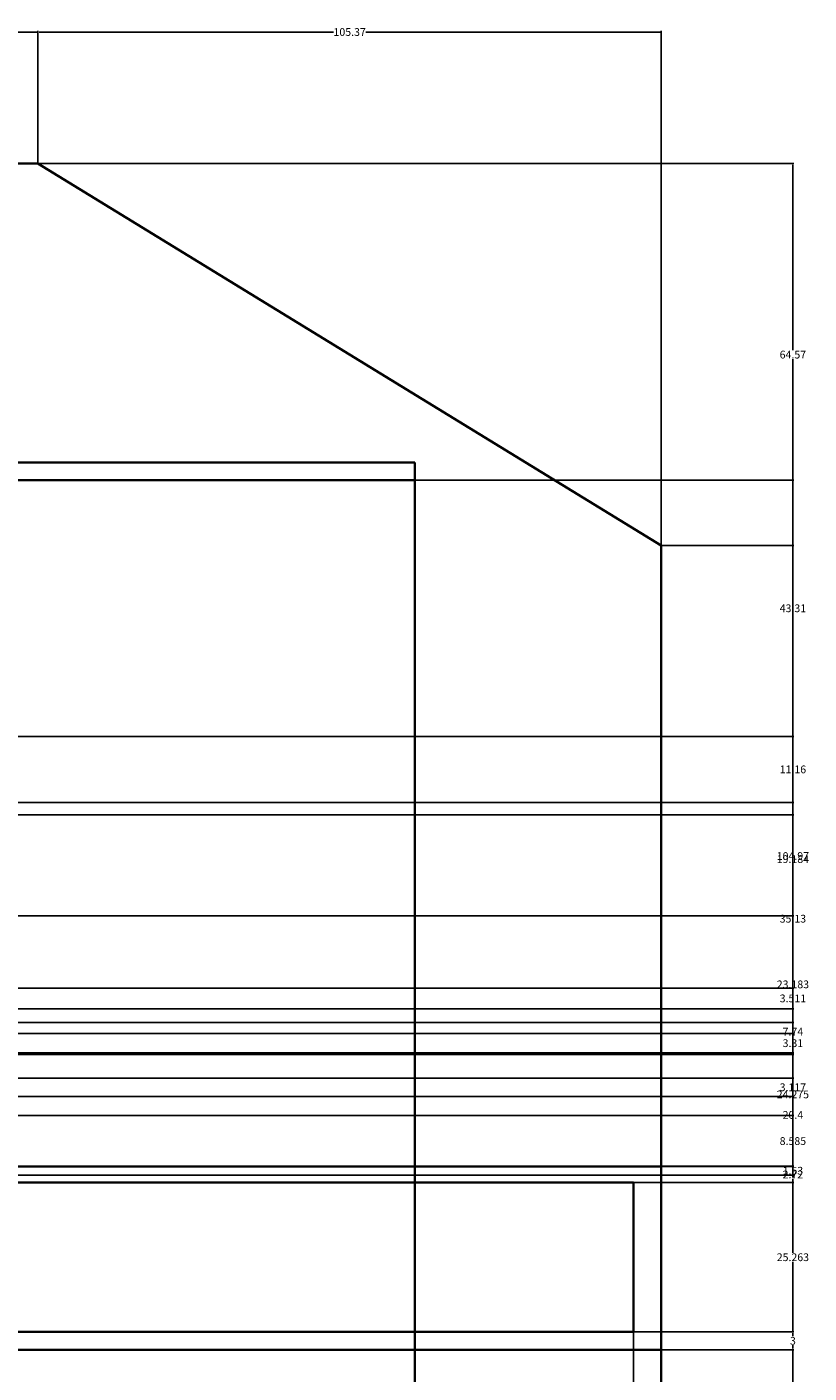
# Model space of a CAD drawing. Units: inches. Extents: x 30 to 515, y 94 to 489.
# Tile 7 of 7: x 383 to 515, y 262 to 489. Entities that reach past the tile are written whole.
import ezdxf

# ---------------------------------------------------------------- set-up
doc = ezdxf.new("R2010")
doc.units = ezdxf.units.IN
doc.header["$MEASUREMENT"] = 0
for name, color, linetype, lineweight in [('A-ANNO-DIMS', 2, 'Continuous', 18), ('A-ROOF', 1, 'Continuous', 35), ('A-WALL', 7, 'Continuous', 35)]:
    doc.layers.add(name, color=color, linetype=linetype, lineweight=lineweight)
doc.styles.get("Standard").update_dxf_attribs({"font": 'arial.ttf'})
doc.dimstyles.get("Standard").update_dxf_attribs({"dimtxt": 1.3125, "dimasz": 0.18, "dimexe": 0.18, "dimexo": 0.0625, "dimgap": 0.09, "dimtad": 0, "dimtih": 1, "dimtoh": 1, "dimdec": 4, "dimzin": 0, "dimdsep": 46, "dimlunit": 4, "dimtxsty": 'Standard', "dimcen": 0.09, "dimadec": 0, "dimazin": 0, "dimtfac": 1, "dimtdec": 4, "dimtofl": 0, "dimtmove": 0, "dimatfit": 3, "dimfxl": 1, "dimtolj": 1, "dimtzin": 0, "dimarcsym": 0})

# ---------------------------------------------------------------- blocks, each defined once
blk = doc.blocks.new('*D5')
at = {"layer": 'A-ANNO-DIMS', "color": 0, "lineweight": -2, "transparency": 16777216}
for p, q in [((191.21, 466.11), (191.21, 488.48)), ((191.39, 488.3), (285.04, 488.3)), ((384.19, 488.3), (290.54, 488.3)), ((384.37, 466.11), (384.37, 488.48))]:
    blk.add_line(p, q, dxfattribs=at)
at = {"layer": 'A-ANNO-DIMS', "color": 0, "transparency": 16777216}
for points in [[(191.39, 488.33), (191.39, 488.27), (191.21, 488.3)], [(384.19, 488.33), (384.19, 488.27), (384.37, 488.3)]]:
    blk.add_solid(points, dxfattribs=at)
at = {"layer": 'Defpoints', "color": 0, "transparency": 16777216}
for p in [(384.37, 488.3), (191.21, 466.05), (384.37, 466.05)]:
    blk.add_point(p, dxfattribs=at)
at = {"layer": 'A-ANNO-DIMS', "color": 0, "transparency": 16777216, "insert": (287.79, 488.3), "char_height": 1.312, "attachment_point": 5}
blk.add_mtext('\\A1;193.16', dxfattribs=at)
blk = doc.blocks.new('*D6')
at = {"layer": 'A-ANNO-DIMS', "color": 0, "lineweight": -2, "transparency": 16777216}
for p, q in [((384.37, 466.11), (384.37, 488.48)), ((384.55, 488.3), (434.3, 488.3)), ((489.56, 488.3), (439.81, 488.3)), ((489.74, 401.54), (489.74, 488.48))]:
    blk.add_line(p, q, dxfattribs=at)
at = {"layer": 'A-ANNO-DIMS', "color": 0, "transparency": 16777216}
for points in [[(384.55, 488.33), (384.55, 488.27), (384.37, 488.3)], [(489.56, 488.33), (489.56, 488.27), (489.74, 488.3)]]:
    blk.add_solid(points, dxfattribs=at)
at = {"layer": 'Defpoints', "color": 0, "transparency": 16777216}
for p in [(489.74, 488.3), (384.37, 466.05), (489.74, 401.48)]:
    blk.add_point(p, dxfattribs=at)
at = {"layer": 'A-ANNO-DIMS', "color": 0, "transparency": 16777216, "insert": (437.06, 488.3), "char_height": 1.312, "attachment_point": 5}
blk.add_mtext('\\A1;105.37', dxfattribs=at)
blk = doc.blocks.new('*D15')
at = {"layer": 'A-ANNO-DIMS', "color": 0, "lineweight": -2, "transparency": 16777216}
for p, q in [((485.027297, 268.465557), (485.027297, 94.504382)), ((489.742649, 265.465557), (489.742649, 94.504382)), ((484.847297, 94.684382), (484.667297, 94.684382)), ((489.922649, 94.684382), (490.102649, 94.684382))]:
    blk.add_line(p, q, dxfattribs=at)
at = {"layer": 'A-ANNO-DIMS', "color": 0, "transparency": 16777216}
for points in [[(484.847297, 94.714382), (484.847297, 94.654382), (485.027297, 94.684382)], [(489.922649, 94.714382), (489.922649, 94.654382), (489.742649, 94.684382)]]:
    blk.add_solid(points, dxfattribs=at)
at = {"layer": 'Defpoints', "color": 0, "transparency": 16777216}
for p in [(485.027297, 268.528057), (489.742649, 265.528057), (489.742649, 94.684382)]:
    blk.add_point(p, dxfattribs=at)
at = {"layer": 'A-ANNO-DIMS', "color": 0, "transparency": 16777216, "insert": (487.384973, 94.684382), "char_height": 1.3125, "attachment_point": 5}
blk.add_mtext('\\A1;4.715', dxfattribs=at)
blk = doc.blocks.new('*D17')
at = {"layer": 'A-ANNO-DIMS', "color": 0, "lineweight": -2, "transparency": 16777216}
for p, q in [((489.81, 265.53), (512.17, 265.53)), ((511.99, 265.35), (511.99, 253.49)), ((511.99, 240.11), (511.99, 251.97)), ((489.81, 239.93), (512.17, 239.93))]:
    blk.add_line(p, q, dxfattribs=at)
at = {"layer": 'A-ANNO-DIMS', "color": 0, "transparency": 16777216}
for points in [[(511.96, 265.35), (512.02, 265.35), (511.99, 265.53)], [(511.96, 240.11), (512.02, 240.11), (511.99, 239.93)]]:
    blk.add_solid(points, dxfattribs=at)
at = {"layer": 'Defpoints', "color": 0, "transparency": 16777216}
for p in [(489.74, 265.53), (511.99, 265.53), (489.74, 239.93)]:
    blk.add_point(p, dxfattribs=at)
at = {"layer": 'A-ANNO-DIMS', "color": 0, "transparency": 16777216, "insert": (511.99, 252.73), "char_height": 1.312, "attachment_point": 5}
blk.add_mtext('\\A1;25.595', dxfattribs=at)
blk = doc.blocks.new('*D18')
at = {"layer": 'A-ANNO-DIMS', "color": 0, "lineweight": -2, "transparency": 16777216}
for p, q in [((485.09, 268.53), (512.17, 268.53)), ((511.99, 268.35), (511.99, 267.79)), ((489.81, 265.53), (512.17, 265.53)), ((511.99, 265.71), (511.99, 266.27))]:
    blk.add_line(p, q, dxfattribs=at)
at = {"layer": 'A-ANNO-DIMS', "color": 0, "transparency": 16777216}
for points in [[(511.96, 268.35), (512.02, 268.35), (511.99, 268.53)], [(511.96, 265.71), (512.02, 265.71), (511.99, 265.53)]]:
    blk.add_solid(points, dxfattribs=at)
at = {"layer": 'Defpoints', "color": 0, "transparency": 16777216}
for p in [(485.03, 268.53), (511.99, 268.53), (489.74, 265.53)]:
    blk.add_point(p, dxfattribs=at)
at = {"layer": 'A-ANNO-DIMS', "color": 0, "transparency": 16777216, "insert": (511.99, 267.03), "char_height": 1.312, "attachment_point": 5}
blk.add_mtext('\\A1;3', dxfattribs=at)
blk = doc.blocks.new('*D19')
at = {"layer": 'A-ANNO-DIMS', "color": 0, "lineweight": -2, "transparency": 16777216}
for p, q in [((485.09, 293.79), (512.17, 293.79)), ((511.99, 293.61), (511.99, 281.92)), ((511.99, 268.71), (511.99, 280.4)), ((485.09, 268.53), (512.17, 268.53))]:
    blk.add_line(p, q, dxfattribs=at)
at = {"layer": 'A-ANNO-DIMS', "color": 0, "transparency": 16777216}
for points in [[(511.96, 293.61), (512.02, 293.61), (511.99, 293.79)], [(511.96, 268.71), (512.02, 268.71), (511.99, 268.53)]]:
    blk.add_solid(points, dxfattribs=at)
at = {"layer": 'Defpoints', "color": 0, "transparency": 16777216}
for p in [(485.03, 293.79), (511.99, 293.79), (485.03, 268.53)]:
    blk.add_point(p, dxfattribs=at)
at = {"layer": 'A-ANNO-DIMS', "color": 0, "transparency": 16777216, "insert": (511.99, 281.16), "char_height": 1.312, "attachment_point": 5}
blk.add_mtext('\\A1;25.263', dxfattribs=at)
blk = doc.blocks.new('*D20')
at = {"layer": 'A-ANNO-DIMS', "color": 0, "lineweight": -2, "transparency": 16777216}
for p, q in [((489.81, 296.51), (512.17, 296.51)), ((511.99, 296.33), (511.99, 295.9)), ((485.09, 293.79), (512.17, 293.79)), ((511.99, 293.97), (511.99, 294.4))]:
    blk.add_line(p, q, dxfattribs=at)
at = {"layer": 'A-ANNO-DIMS', "color": 0, "transparency": 16777216}
for points in [[(511.96, 296.33), (512.02, 296.33), (511.99, 296.51)], [(511.96, 293.97), (512.02, 293.97), (511.99, 293.79)]]:
    blk.add_solid(points, dxfattribs=at)
at = {"layer": 'Defpoints', "color": 0, "transparency": 16777216}
for p in [(489.74, 296.51), (511.99, 296.51), (485.03, 293.79)]:
    blk.add_point(p, dxfattribs=at)
at = {"layer": 'A-ANNO-DIMS', "color": 0, "transparency": 16777216, "insert": (511.99, 295.15), "char_height": 1.312, "attachment_point": 5}
blk.add_mtext('\\A1;2.72', dxfattribs=at)
blk = doc.blocks.new('*D21')
at = {"layer": 'A-ANNO-DIMS', "color": 0, "lineweight": -2, "transparency": 16777216}
for p, q in [((489.81, 401.48), (512.17, 401.48)), ((511.99, 401.3), (511.99, 349.75)), ((511.99, 296.69), (511.99, 348.23)), ((489.81, 296.51), (512.17, 296.51))]:
    blk.add_line(p, q, dxfattribs=at)
at = {"layer": 'A-ANNO-DIMS', "color": 0, "transparency": 16777216}
for points in [[(511.96, 401.3), (512.02, 401.3), (511.99, 401.48)], [(511.96, 296.69), (512.02, 296.69), (511.99, 296.51)]]:
    blk.add_solid(points, dxfattribs=at)
at = {"layer": 'Defpoints', "color": 0, "transparency": 16777216}
for p in [(489.74, 401.48), (511.99, 401.48), (489.74, 296.51)]:
    blk.add_point(p, dxfattribs=at)
at = {"layer": 'A-ANNO-DIMS', "color": 0, "transparency": 16777216, "insert": (511.99, 348.99), "char_height": 1.312, "attachment_point": 5}
blk.add_mtext('\\A1;104.97', dxfattribs=at)
blk = doc.blocks.new('*D22')
at = {"layer": 'A-ANNO-DIMS', "color": 0, "lineweight": -2, "transparency": 16777216}
for p, q in [((384.43, 466.05), (512.17, 466.05)), ((511.99, 465.87), (511.99, 434.53)), ((511.99, 401.66), (511.99, 433)), ((489.81, 401.48), (512.17, 401.48))]:
    blk.add_line(p, q, dxfattribs=at)
at = {"layer": 'A-ANNO-DIMS', "color": 0, "transparency": 16777216}
for points in [[(511.96, 465.87), (512.02, 465.87), (511.99, 466.05)], [(511.96, 401.66), (512.02, 401.66), (511.99, 401.48)]]:
    blk.add_solid(points, dxfattribs=at)
at = {"layer": 'Defpoints', "color": 0, "transparency": 16777216}
for p in [(384.37, 466.05), (511.99, 466.05), (489.74, 401.48)]:
    blk.add_point(p, dxfattribs=at)
at = {"layer": 'A-ANNO-DIMS', "color": 0, "transparency": 16777216, "insert": (511.99, 433.76), "char_height": 1.312, "attachment_point": 5}
blk.add_mtext('\\A1;64.57', dxfattribs=at)
blk = doc.blocks.new('*D30')
at = {"layer": 'A-ANNO-DIMS', "color": 0, "lineweight": -2, "transparency": 16777216}
for p, q in [((210.86, 412.53), (512.17, 412.53)), ((511.99, 412.35), (511.99, 391.63)), ((511.99, 369.4), (511.99, 390.11)), ((247.77, 369.22), (512.17, 369.22))]:
    blk.add_line(p, q, dxfattribs=at)
at = {"layer": 'A-ANNO-DIMS', "color": 0, "transparency": 16777216}
for points in [[(511.96, 412.35), (512.02, 412.35), (511.99, 412.53)], [(511.96, 369.4), (512.02, 369.4), (511.99, 369.22)]]:
    blk.add_solid(points, dxfattribs=at)
at = {"layer": 'Defpoints', "color": 0, "transparency": 16777216}
for p in [(210.8, 412.53), (511.99, 412.53), (247.71, 369.22)]:
    blk.add_point(p, dxfattribs=at)
at = {"layer": 'A-ANNO-DIMS', "color": 0, "transparency": 16777216, "insert": (511.99, 390.87), "char_height": 1.312, "attachment_point": 5}
blk.add_mtext('\\A1;43.31', dxfattribs=at)
blk = doc.blocks.new('*D59')
at = {"layer": 'A-ANNO-DIMS', "color": 0, "lineweight": -2, "transparency": 16777216}
for p, q in [((193.04, 296.55), (512.17, 296.55)), ((511.99, 296.73), (511.99, 296.91)), ((195.76, 295.02), (512.17, 295.02)), ((511.99, 294.84), (511.99, 294.66))]:
    blk.add_line(p, q, dxfattribs=at)
at = {"layer": 'A-ANNO-DIMS', "color": 0, "transparency": 16777216}
for points in [[(511.96, 296.73), (512.02, 296.73), (511.99, 296.55)], [(511.96, 294.84), (512.02, 294.84), (511.99, 295.02)]]:
    blk.add_solid(points, dxfattribs=at)
at = {"layer": 'Defpoints', "color": 0, "transparency": 16777216}
for p in [(192.98, 296.55), (511.99, 296.55), (195.7, 295.02)]:
    blk.add_point(p, dxfattribs=at)
at = {"layer": 'A-ANNO-DIMS', "color": 0, "transparency": 16777216, "insert": (511.99, 295.78), "char_height": 1.312, "attachment_point": 5}
blk.add_mtext('\\A1;1.53', dxfattribs=at)
blk = doc.blocks.new('*D60')
at = {"layer": 'A-ANNO-DIMS', "color": 0, "lineweight": -2, "transparency": 16777216}
for p, q in [((191.31, 320.83), (512.17, 320.83)), ((511.99, 320.65), (511.99, 309.45)), ((511.99, 296.73), (511.99, 307.93)), ((193.04, 296.55), (512.17, 296.55))]:
    blk.add_line(p, q, dxfattribs=at)
at = {"layer": 'A-ANNO-DIMS', "color": 0, "transparency": 16777216}
for points in [[(511.96, 320.65), (512.02, 320.65), (511.99, 320.83)], [(511.96, 296.73), (512.02, 296.73), (511.99, 296.55)]]:
    blk.add_solid(points, dxfattribs=at)
at = {"layer": 'Defpoints', "color": 0, "transparency": 16777216}
for p in [(191.25, 320.83), (511.99, 320.83), (192.98, 296.55)]:
    blk.add_point(p, dxfattribs=at)
at = {"layer": 'A-ANNO-DIMS', "color": 0, "transparency": 16777216, "insert": (511.99, 308.69), "char_height": 1.312, "attachment_point": 5}
blk.add_mtext('\\A1;24.275', dxfattribs=at)
blk = doc.blocks.new('*D61')
at = {"layer": 'A-ANNO-DIMS', "color": 0, "lineweight": -2, "transparency": 16777216}
for p, q in [((193.04, 355.95), (512.17, 355.95)), ((511.99, 355.77), (511.99, 339.15)), ((511.99, 321.01), (511.99, 337.63)), ((191.31, 320.83), (512.17, 320.83))]:
    blk.add_line(p, q, dxfattribs=at)
at = {"layer": 'A-ANNO-DIMS', "color": 0, "transparency": 16777216}
for points in [[(511.96, 355.77), (512.02, 355.77), (511.99, 355.95)], [(511.96, 321.01), (512.02, 321.01), (511.99, 320.83)]]:
    blk.add_solid(points, dxfattribs=at)
at = {"layer": 'Defpoints', "color": 0, "transparency": 16777216}
for p in [(192.98, 355.95), (511.99, 355.95), (191.25, 320.83)]:
    blk.add_point(p, dxfattribs=at)
at = {"layer": 'A-ANNO-DIMS', "color": 0, "transparency": 16777216, "insert": (511.99, 338.39), "char_height": 1.312, "attachment_point": 5}
blk.add_mtext('\\A1;35.13', dxfattribs=at)
blk = doc.blocks.new('*D62')
at = {"layer": 'A-ANNO-DIMS', "color": 0, "lineweight": -2, "transparency": 16777216}
for p, q in [((195.76, 315.42), (512.17, 315.42)), ((511.99, 315.24), (511.99, 305.98)), ((511.99, 295.2), (511.99, 304.46)), ((195.76, 295.02), (512.17, 295.02))]:
    blk.add_line(p, q, dxfattribs=at)
at = {"layer": 'A-ANNO-DIMS', "color": 0, "transparency": 16777216}
for points in [[(511.96, 315.24), (512.02, 315.24), (511.99, 315.42)], [(511.96, 295.2), (512.02, 295.2), (511.99, 295.02)]]:
    blk.add_solid(points, dxfattribs=at)
at = {"layer": 'Defpoints', "color": 0, "transparency": 16777216}
for p in [(195.7, 315.42), (511.99, 315.42), (195.7, 295.02)]:
    blk.add_point(p, dxfattribs=at)
at = {"layer": 'A-ANNO-DIMS', "color": 0, "transparency": 16777216, "insert": (511.99, 305.22), "char_height": 1.312, "attachment_point": 5}
blk.add_mtext('\\A1;20.4', dxfattribs=at)
blk = doc.blocks.new('*D63')
at = {"layer": 'A-ANNO-DIMS', "color": 0, "lineweight": -2, "transparency": 16777216}
for p, q in [((195.76, 323.16), (512.17, 323.16)), ((511.99, 322.98), (511.99, 320.04)), ((511.99, 315.6), (511.99, 318.54)), ((195.76, 315.42), (512.17, 315.42))]:
    blk.add_line(p, q, dxfattribs=at)
at = {"layer": 'A-ANNO-DIMS', "color": 0, "transparency": 16777216}
for points in [[(511.96, 322.98), (512.02, 322.98), (511.99, 323.16)], [(511.96, 315.6), (512.02, 315.6), (511.99, 315.42)]]:
    blk.add_solid(points, dxfattribs=at)
at = {"layer": 'Defpoints', "color": 0, "transparency": 16777216}
for p in [(195.7, 323.16), (511.99, 323.16), (195.7, 315.42)]:
    blk.add_point(p, dxfattribs=at)
at = {"layer": 'A-ANNO-DIMS', "color": 0, "transparency": 16777216, "insert": (511.99, 319.29), "char_height": 1.312, "attachment_point": 5}
blk.add_mtext('\\A1;7.74', dxfattribs=at)
blk = doc.blocks.new('*D64')
at = {"layer": 'A-ANNO-DIMS', "color": 0, "lineweight": -2, "transparency": 16777216}
for p, q in [((195.76, 326.67), (512.17, 326.67)), ((511.99, 326.49), (511.99, 325.68)), ((511.99, 323.34), (511.99, 324.16)), ((195.76, 323.16), (512.17, 323.16))]:
    blk.add_line(p, q, dxfattribs=at)
at = {"layer": 'A-ANNO-DIMS', "color": 0, "transparency": 16777216}
for points in [[(511.96, 326.49), (512.02, 326.49), (511.99, 326.67)], [(511.96, 323.34), (512.02, 323.34), (511.99, 323.16)]]:
    blk.add_solid(points, dxfattribs=at)
at = {"layer": 'Defpoints', "color": 0, "transparency": 16777216}
for p in [(195.7, 326.67), (511.99, 326.67), (195.7, 323.16)]:
    blk.add_point(p, dxfattribs=at)
at = {"layer": 'A-ANNO-DIMS', "color": 0, "transparency": 16777216, "insert": (511.99, 324.92), "char_height": 1.312, "attachment_point": 5}
blk.add_mtext('\\A1;3.511', dxfattribs=at)
blk = doc.blocks.new('*D71')
at = {"layer": 'A-ANNO-DIMS', "color": 0, "lineweight": -2, "transparency": 16777216}
for p, q in [((380.69, 305.1), (512.17, 305.1)), ((511.99, 304.92), (511.99, 301.56)), ((511.99, 296.69), (511.99, 300.04)), ((380.69, 296.51), (512.17, 296.51))]:
    blk.add_line(p, q, dxfattribs=at)
at = {"layer": 'A-ANNO-DIMS', "color": 0, "transparency": 16777216}
for points in [[(511.96, 304.92), (512.02, 304.92), (511.99, 305.1)], [(511.96, 296.69), (512.02, 296.69), (511.99, 296.51)]]:
    blk.add_solid(points, dxfattribs=at)
at = {"layer": 'Defpoints', "color": 0, "transparency": 16777216}
for p in [(380.63, 305.1), (511.99, 305.1), (380.63, 296.51)]:
    blk.add_point(p, dxfattribs=at)
at = {"layer": 'A-ANNO-DIMS', "color": 0, "transparency": 16777216, "insert": (511.99, 300.8), "char_height": 1.312, "attachment_point": 5}
blk.add_mtext('\\A1;8.585', dxfattribs=at)
blk = doc.blocks.new('*D72')
at = {"layer": 'A-ANNO-DIMS', "color": 0, "lineweight": -2, "transparency": 16777216}
for p, q in [((380.69, 311.45), (512.17, 311.45)), ((511.99, 311.27), (511.99, 310.65)), ((380.69, 308.33), (512.17, 308.33)), ((511.99, 308.51), (511.99, 309.13))]:
    blk.add_line(p, q, dxfattribs=at)
at = {"layer": 'A-ANNO-DIMS', "color": 0, "transparency": 16777216}
for points in [[(511.96, 311.27), (512.02, 311.27), (511.99, 311.45)], [(511.96, 308.51), (512.02, 308.51), (511.99, 308.33)]]:
    blk.add_solid(points, dxfattribs=at)
at = {"layer": 'Defpoints', "color": 0, "transparency": 16777216}
for p in [(380.63, 311.45), (511.99, 311.45), (380.63, 308.33)]:
    blk.add_point(p, dxfattribs=at)
at = {"layer": 'A-ANNO-DIMS', "color": 0, "transparency": 16777216, "insert": (511.99, 309.89), "char_height": 1.312, "attachment_point": 5}
blk.add_mtext('\\A1;3.117', dxfattribs=at)
blk = doc.blocks.new('*D73')
at = {"layer": 'A-ANNO-DIMS', "color": 0, "lineweight": -2, "transparency": 16777216}
for p, q in [((380.69, 319), (512.17, 319)), ((511.99, 318.82), (511.99, 318.11)), ((511.99, 315.87), (511.99, 316.59)), ((380.69, 315.69), (512.17, 315.69))]:
    blk.add_line(p, q, dxfattribs=at)
at = {"layer": 'A-ANNO-DIMS', "color": 0, "transparency": 16777216}
for points in [[(511.96, 318.82), (512.02, 318.82), (511.99, 319)], [(511.96, 315.87), (512.02, 315.87), (511.99, 315.69)]]:
    blk.add_solid(points, dxfattribs=at)
at = {"layer": 'Defpoints', "color": 0, "transparency": 16777216}
for p in [(380.63, 319), (511.99, 319), (380.63, 315.69)]:
    blk.add_point(p, dxfattribs=at)
at = {"layer": 'A-ANNO-DIMS', "color": 0, "transparency": 16777216, "insert": (511.99, 317.35), "char_height": 1.312, "attachment_point": 5}
blk.add_mtext('\\A1;3.31', dxfattribs=at)
blk = doc.blocks.new('*D74')
at = {"layer": 'A-ANNO-DIMS', "color": 0, "lineweight": -2, "transparency": 16777216}
for p, q in [((380.69, 326.67), (512.17, 326.67)), ((511.99, 326.49), (511.99, 325.68)), ((511.99, 323.34), (511.99, 324.16)), ((380.69, 323.16), (512.17, 323.16))]:
    blk.add_line(p, q, dxfattribs=at)
at = {"layer": 'A-ANNO-DIMS', "color": 0, "transparency": 16777216}
for points in [[(511.96, 326.49), (512.02, 326.49), (511.99, 326.67)], [(511.96, 323.34), (512.02, 323.34), (511.99, 323.16)]]:
    blk.add_solid(points, dxfattribs=at)
at = {"layer": 'Defpoints', "color": 0, "transparency": 16777216}
for p in [(380.63, 326.67), (511.99, 326.67), (380.63, 323.16)]:
    blk.add_point(p, dxfattribs=at)
at = {"layer": 'A-ANNO-DIMS', "color": 0, "transparency": 16777216, "insert": (511.99, 324.92), "char_height": 1.312, "attachment_point": 5}
blk.add_mtext('\\A1;3.511', dxfattribs=at)
blk = doc.blocks.new('*D78')
at = {"layer": 'A-ANNO-DIMS', "color": 0, "lineweight": -2, "transparency": 16777216}
for p, q in [((245.42, 338.88), (512.17, 338.88)), ((511.99, 338.7), (511.99, 328.05)), ((511.99, 315.87), (511.99, 326.52)), ((247.77, 315.69), (512.17, 315.69))]:
    blk.add_line(p, q, dxfattribs=at)
at = {"layer": 'A-ANNO-DIMS', "color": 0, "transparency": 16777216}
for points in [[(511.96, 338.7), (512.02, 338.7), (511.99, 338.88)], [(511.96, 315.87), (512.02, 315.87), (511.99, 315.69)]]:
    blk.add_solid(points, dxfattribs=at)
at = {"layer": 'Defpoints', "color": 0, "transparency": 16777216}
for p in [(245.35, 338.88), (511.99, 338.88), (247.71, 315.69)]:
    blk.add_point(p, dxfattribs=at)
at = {"layer": 'A-ANNO-DIMS', "color": 0, "transparency": 16777216, "insert": (511.99, 327.29), "char_height": 1.312, "attachment_point": 5}
blk.add_mtext('\\A1;23.183', dxfattribs=at)
blk = doc.blocks.new('*D79')
at = {"layer": 'A-ANNO-DIMS', "color": 0, "lineweight": -2, "transparency": 16777216}
for p, q in [((247.77, 358.06), (512.17, 358.06)), ((511.99, 357.88), (511.99, 349.23)), ((511.99, 339.06), (511.99, 347.71)), ((245.42, 338.88), (512.17, 338.88))]:
    blk.add_line(p, q, dxfattribs=at)
at = {"layer": 'A-ANNO-DIMS', "color": 0, "transparency": 16777216}
for points in [[(511.96, 357.88), (512.02, 357.88), (511.99, 358.06)], [(511.96, 339.06), (512.02, 339.06), (511.99, 338.88)]]:
    blk.add_solid(points, dxfattribs=at)
at = {"layer": 'Defpoints', "color": 0, "transparency": 16777216}
for p in [(247.71, 358.06), (511.99, 358.06), (245.35, 338.88)]:
    blk.add_point(p, dxfattribs=at)
at = {"layer": 'A-ANNO-DIMS', "color": 0, "transparency": 16777216, "insert": (511.99, 348.47), "char_height": 1.312, "attachment_point": 5}
blk.add_mtext('\\A1;19.184', dxfattribs=at)
blk = doc.blocks.new('*D80')
at = {"layer": 'A-ANNO-DIMS', "color": 0, "lineweight": -2, "transparency": 16777216}
for p, q in [((247.77, 369.22), (512.17, 369.22)), ((511.99, 369.04), (511.99, 364.4)), ((511.99, 358.24), (511.99, 362.88)), ((247.77, 358.06), (512.17, 358.06))]:
    blk.add_line(p, q, dxfattribs=at)
at = {"layer": 'A-ANNO-DIMS', "color": 0, "transparency": 16777216}
for points in [[(511.96, 369.04), (512.02, 369.04), (511.99, 369.22)], [(511.96, 358.24), (512.02, 358.24), (511.99, 358.06)]]:
    blk.add_solid(points, dxfattribs=at)
at = {"layer": 'Defpoints', "color": 0, "transparency": 16777216}
for p in [(247.71, 369.22), (511.99, 369.22), (247.71, 358.06)]:
    blk.add_point(p, dxfattribs=at)
at = {"layer": 'A-ANNO-DIMS', "color": 0, "transparency": 16777216, "insert": (511.99, 363.64), "char_height": 1.312, "attachment_point": 5}
blk.add_mtext('\\A1;11.16', dxfattribs=at)

msp = doc.modelspace()

# ---------------------------------------------------------------- linework, layer by layer
at = {"layer": 'A-ROOF'}
for p, q in [((337.6614, 466.0503), (384.3704, 466.0503)), ((384.3704, 466.0503), (489.7426, 401.4795)), ((489.7426, 401.4795), (489.7426, 239.9328))]:
    msp.add_line(p, q, dxfattribs=at)
at = {"layer": 'A-WALL'}
for p, q in [((67.017, 415.5281), (448.0511, 415.5281)), ((448.0511, 415.5281), (448.0511, 412.5281)), ((210.8018, 412.5281), (448.0511, 412.5281)), ((448.0511, 268.5281), (448.0511, 412.5281)), ((489.7426, 296.5098), (210.8018, 296.5098)), ((489.7426, 265.5281), (489.7426, 296.5098)), ((485.0273, 293.7914), (207.9863, 293.7914)), ((485.0273, 268.5281), (485.0273, 293.7914)), ((67.017, 268.5281), (448.0511, 268.5281)), ((448.0511, 268.5281), (448.0511, 265.5281)), ((448.0511, 268.5281), (485.0273, 268.5281)), ((67.017, 265.5281), (448.0511, 265.5281)), ((448.0511, 265.5281), (448.0511, 121.5281)), ((448.0511, 265.5281), (485.6625, 265.5281)), ((485.6625, 265.5281), (489.7426, 265.5281))]:
    msp.add_line(p, q, dxfattribs=at)

# ---------------------------------------------------------------- dimensions: what is measured, and where the dimension line sits
at = {"layer": 'A-ANNO-DIMS'}
for base, p1, p2, override, picture, middle in [((384.3704, 488.3003), (191.2145, 466.0503), (384.3704, 466.0503), {"dimdec": 2, "dimlfac": 1, "dimrnd": 0, "dimzin": 0, "dimdsep": 46, "dimlunit": 2}, '*D5', (287.7924, 488.3003)), ((489.7426, 488.3003), (384.3704, 466.0503), (489.7426, 401.4795), {"dimdec": 2, "dimlfac": 1, "dimrnd": 0, "dimzin": 0, "dimdsep": 46, "dimlunit": 2}, '*D6', (437.0565, 488.3003)), ((489.7426, 94.6844), (485.0273, 268.5281), (489.7426, 265.5281), {"dimdec": 3, "dimlfac": 1, "dimrnd": 0, "dimzin": 0, "dimdsep": 46, "dimlunit": 2}, '*D15', (487.385, 94.6844))]:
    dim = msp.add_linear_dim(base=base, p1=p1, p2=p2, dimstyle='Standard', override=override, dxfattribs=at)
    dim.commit()
    dim.dimension.update_dxf_attribs({"geometry": picture, "text_midpoint": middle})
for base, p1, p2, override, picture, middle in [((511.9926, 466.0503), (489.7426, 401.4795), (384.3704, 466.0503), {"dimdec": 2, "dimlfac": 1, "dimrnd": 0, "dimzin": 0, "dimdsep": 46, "dimlunit": 2}, '*D22', (511.9926, 433.7649)), ((511.9926, 412.5281), (247.7111, 369.2198), (210.8018, 412.5281), {"dimdec": 2, "dimlfac": 1, "dimrnd": 0, "dimzin": 0, "dimdsep": 46, "dimlunit": 2}, '*D30', (511.9926, 390.8739)), ((511.9926, 401.4795), (489.7426, 296.5098), (489.7426, 401.4795), {"dimdec": 2, "dimlfac": 1, "dimrnd": 0, "dimzin": 0, "dimdsep": 46, "dimlunit": 2}, '*D21', (511.9926, 348.9947)), ((511.9926, 369.2198), (247.7111, 358.0606), (247.7111, 369.2198), {"dimdec": 2, "dimlfac": 1, "dimrnd": 0, "dimzin": 0, "dimdsep": 46, "dimlunit": 2}, '*D80', (511.9926, 363.6402)), ((511.9926, 358.0606), (245.3541, 338.8769), (247.7111, 358.0606), {"dimdec": 3, "dimlfac": 1, "dimrnd": 0, "dimzin": 0, "dimdsep": 46, "dimlunit": 2}, '*D79', (511.9926, 348.4687)), ((511.9926, 355.9547), (191.2506, 320.8262), (192.9806, 355.9547), {"dimdec": 2, "dimlfac": 1, "dimrnd": 0, "dimzin": 0, "dimdsep": 46, "dimlunit": 2}, '*D61', (511.9926, 338.3905)), ((511.9926, 338.8769), (247.7111, 315.6935), (245.3541, 338.8769), {"dimdec": 3, "dimlfac": 1, "dimrnd": 0, "dimzin": 0, "dimdsep": 46, "dimlunit": 2}, '*D78', (511.9926, 327.2852)), ((511.9926, 326.6711), (195.6952, 323.1601), (195.6952, 326.6711), {"dimdec": 3, "dimlfac": 1, "dimrnd": 0, "dimzin": 0, "dimdsep": 46, "dimlunit": 2}, '*D64', (511.9926, 324.9156)), ((511.9926, 326.6711), (380.6303, 323.1601), (380.6303, 326.6711), {"dimdec": 3, "dimlfac": 1, "dimrnd": 0, "dimzin": 0, "dimdsep": 46, "dimlunit": 2}, '*D74', (511.9926, 324.9156)), ((511.9926, 323.1601), (195.6952, 315.4195), (195.6952, 323.1601), {"dimdec": 2, "dimlfac": 1, "dimrnd": 0, "dimzin": 0, "dimdsep": 46, "dimlunit": 2}, '*D63', (511.9926, 319.2898)), ((511.9926, 320.8262), (192.9806, 296.551), (191.2506, 320.8262), {"dimdec": 3, "dimlfac": 1, "dimrnd": 0, "dimzin": 0, "dimdsep": 46, "dimlunit": 2}, '*D60', (511.9926, 308.6886)), ((511.9926, 319.0036), (380.6303, 315.6935), (380.6303, 319.0036), {"dimdec": 2, "dimlfac": 1, "dimrnd": 0, "dimzin": 0, "dimdsep": 46, "dimlunit": 2}, '*D73', (511.9926, 317.3485)), ((511.9926, 315.4195), (195.6952, 295.0176), (195.6952, 315.4195), {"dimdec": 1, "dimlfac": 1, "dimrnd": 0, "dimzin": 0, "dimdsep": 46, "dimlunit": 2}, '*D62', (511.9926, 305.2186)), ((511.9926, 311.4502), (380.6303, 308.3335), (380.6303, 311.4502), {"dimdec": 3, "dimlfac": 1, "dimrnd": 0, "dimzin": 0, "dimdsep": 46, "dimlunit": 2}, '*D72', (511.9926, 309.8918)), ((511.9926, 305.0952), (380.6303, 296.5098), (380.6303, 305.0952), {"dimdec": 3, "dimlfac": 1, "dimrnd": 0, "dimzin": 0, "dimdsep": 46, "dimlunit": 2}, '*D71', (511.9926, 300.8025)), ((511.9926, 296.551), (195.6952, 295.0176), (192.9806, 296.551), {"dimdec": 2, "dimlfac": 1, "dimrnd": 0, "dimzin": 0, "dimdsep": 46, "dimlunit": 2}, '*D59', (511.9926, 295.7843)), ((511.9926, 296.5098), (485.0273, 293.7914), (489.7426, 296.5098), {"dimdec": 2, "dimlfac": 1, "dimrnd": 0, "dimzin": 0, "dimdsep": 46, "dimlunit": 2}, '*D20', (511.9926, 295.1506)), ((511.9926, 293.7914), (485.0273, 268.5281), (485.0273, 293.7914), {"dimdec": 3, "dimlfac": 1, "dimrnd": 0, "dimzin": 0, "dimdsep": 46, "dimlunit": 2}, '*D19', (511.9926, 281.1597)), ((511.9926, 268.5281), (489.7426, 265.5281), (485.0273, 268.5281), {"dimdec": 0, "dimlfac": 1, "dimrnd": 0, "dimzin": 0, "dimdsep": 46, "dimlunit": 2}, '*D18', (511.9926, 267.0281)), ((511.9926, 265.5281), (489.7426, 239.9328), (489.7426, 265.5281), {"dimdec": 3, "dimlfac": 1, "dimrnd": 0, "dimzin": 0, "dimdsep": 46, "dimlunit": 2}, '*D17', (511.9926, 252.7304))]:
    dim = msp.add_linear_dim(base=base, p1=p1, p2=p2, angle=90, dimstyle='Standard', override=override, dxfattribs=at)
    dim.commit()
    dim.dimension.update_dxf_attribs({"geometry": picture, "text_midpoint": middle})

doc.saveas('drawing.dxf')
